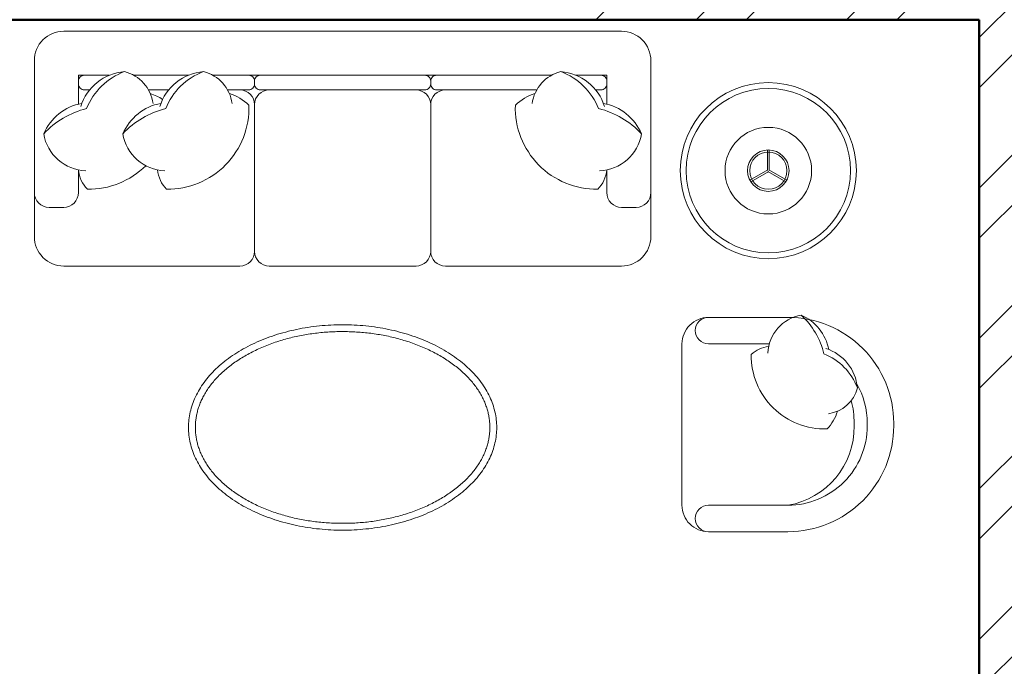
# Model space of a CAD drawing. Units: inches. Extents: x 1901 to 2863, y 888 to 2433.
# Tile 38 of 91: x 2530 to 2618, y 1603 to 1661. Entities that reach past the tile are written whole.
import ezdxf

# ---------------------------------------------------------------- set-up
doc = ezdxf.new("R2010")
doc.units = ezdxf.units.IN
for name, color, linetype, lineweight in [('A-FURN', 8, 'Continuous', 18), ('A-WALL', 7, 'Continuous', 50), ('A-WALL-PATT', 8, 'Continuous', 13)]:
    doc.layers.add(name, color=color, linetype=linetype, lineweight=lineweight)

msp = doc.modelspace()

# ---------------------------------------------------------------- hatches: boundary and pattern name
at = {"layer": 'A-WALL-PATT'}
h = msp.add_hatch(dxfattribs=at)
h.set_pattern_fill('ANSI32', color=256)
h.paths.add_polyline_path([(2443.926, 2139.888), (2439.426, 2139.888), (2439.426, 2069.348), (2441.676, 2069.348), (2443.926, 2069.348), (2443.926, 2078.634), (2521.926, 2078.634), (2521.926, 2075.067), (2524.176, 2075.067), (2526.426, 2075.067), (2526.426, 2078.634), (2571.755, 2078.634), (2571.755, 2080.884), (2571.755, 2083.134), (2443.926, 2083.134)])
h.paths.add_polyline_path([(2526.426, 2054.634), (2524.176, 2054.634), (2521.926, 2054.634), (2521.926, 2030.634), (2443.926, 2030.634), (2443.926, 2045.348), (2439.426, 2045.348), (2439.426, 1983.867), (2443.926, 1983.867), (2443.926, 2026.134), (2521.926, 2026.134), (2526.426, 2026.134)])
h.paths.add_polyline_path([(2443.926, 1923.867), (2439.426, 1923.867), (2439.426, 1872.634), (2443.926, 1872.634)])
h.paths.add_polyline_path([(2636.233, 1766.134), (2609.926, 1766.134), (2609.926, 1779.785), (2605.426, 1779.785), (2605.426, 1766.134), (2486.614, 1766.134), (2486.614, 1770.671), (2482.114, 1770.671), (2482.114, 1766.134), (2482.114, 1761.634), (2636.233, 1761.634), (2636.233, 1763.884)])
h.paths.add_polyline_path([(2519.536, 1663.384), (2519.536, 1665.634), (2494.926, 1665.634), (2481.831, 1665.634), (2481.831, 1663.384), (2481.831, 1661.134), (2490.426, 1661.134), (2490.426, 1640.157), (2494.926, 1640.157), (2494.926, 1661.134), (2519.536, 1661.134)])
h.paths.add_polyline_path([(2443.926, 1712.134), (2443.926, 1716.634), (2414.464, 1716.634), (2414.464, 1712.134), (2439.426, 1712.134), (2439.426, 1545.507), (2443.926, 1545.507), (2443.926, 1661.134), (2448.475, 1661.134), (2448.475, 1665.634), (2443.926, 1665.634)])
h.paths.add_polyline_path([(2343.426, 1712.134), (2365.525, 1712.134), (2365.525, 1714.384), (2365.525, 1716.634), (2333.871, 1716.634), (2333.871, 1714.384), (2333.871, 1712.134), (2338.926, 1712.134), (2338.926, 1575.634), (2338.926, 1545.507), (2343.426, 1545.507), (2343.426, 1547.507), (2343.426, 1580.134)])
h.paths.add_polyline_path([(2752.926, 1665.634), (2579.536, 1665.634), (2579.536, 1661.134), (2615.926, 1661.134), (2615.926, 1529.134), (2598.931, 1529.134), (2598.931, 1524.634), (2623.127, 1524.634), (2623.127, 1526.884), (2623.127, 1529.134), (2620.426, 1529.134), (2620.426, 1661.134), (2748.426, 1661.134), (2748.426, 1633.499), (2752.926, 1633.499)])
h.paths.add_polyline_path([(2752.926, 1419.929), (2748.426, 1419.929), (2748.426, 1400.134), (2659.426, 1400.134), (2659.426, 1444.333), (2657.176, 1444.333), (2654.926, 1444.333), (2654.926, 1400.134), (2643.649, 1400.134), (2643.649, 1395.634), (2748.426, 1395.634), (2748.426, 1364.035), (2752.926, 1364.035)])
h.paths.add_polyline_path([(2752.926, 1492.878), (2748.426, 1492.878), (2748.426, 1476.634), (2667.426, 1476.634), (2667.426, 1479.71), (2665.176, 1479.71), (2662.926, 1479.71), (2662.926, 1476.634), (2654.926, 1476.634), (2654.926, 1469.536), (2659.426, 1469.536), (2659.426, 1472.134), (2748.426, 1472.134), (2748.426, 1455.929), (2752.926, 1455.929)])
h.paths.add_polyline_path([(2752.926, 1304.035), (2748.426, 1304.035), (2748.426, 1263.634), (2738.66, 1263.634), (2738.66, 1259.134), (2752.926, 1259.134)])
h.paths.add_polyline_path([(2685.926, 1259.134), (2695.49, 1259.134), (2695.49, 1261.384), (2695.49, 1263.634), (2677.837, 1263.634), (2677.837, 1261.384), (2677.837, 1259.134), (2681.426, 1259.134), (2681.426, 1203.634), (2653.277, 1203.634), (2653.277, 1199.134), (2685.926, 1199.134), (2685.926, 1203.634)])
h.paths.add_polyline_path([(2609.426, 1395.634), (2611.848, 1395.634), (2611.848, 1400.134), (2598.888, 1400.134), (2598.888, 1397.884), (2598.888, 1395.634), (2604.926, 1395.634), (2604.926, 1268.134), (2554.726, 1268.134), (2554.726, 1265.884), (2554.726, 1263.634), (2604.926, 1263.634), (2604.926, 1203.634), (2571.306, 1203.634), (2571.306, 1199.134), (2604.926, 1199.134), (2629.277, 1199.134), (2629.277, 1201.384), (2629.277, 1203.634), (2609.426, 1203.634), (2609.426, 1258.634), (2609.426, 1259.134), (2654.804, 1259.134), (2654.804, 1263.634), (2609.426, 1263.634)])
h.paths.add_polyline_path([(2443.926, 1304.035), (2439.426, 1304.035), (2439.426, 1259.134), (2443.926, 1259.134), (2456.16, 1259.134), (2456.16, 1261.384), (2456.16, 1263.634), (2443.926, 1263.634)])
h.paths.add_polyline_path([(2525.426, 1263.634), (2531.778, 1263.634), (2531.778, 1268.134), (2520.926, 1268.134), (2520.926, 1263.634), (2511.409, 1263.634), (2511.409, 1259.134), (2520.926, 1259.134), (2520.926, 1199.134), (2547.306, 1199.134), (2547.306, 1201.384), (2547.306, 1203.634), (2525.426, 1203.634)])
h.paths.add_polyline_path([(2443.926, 1434.842), (2439.426, 1434.842), (2439.426, 1364.035), (2441.676, 1364.035), (2443.926, 1364.035)])
h.paths.add_polyline_path([(2567.134, 1400.134), (2443.926, 1400.134), (2443.926, 1395.634), (2567.134, 1395.634)])
h.paths.add_polyline_path([(2443.926, 1545.507), (2439.426, 1545.507), (2439.426, 1494.842), (2443.926, 1494.842)])
h.paths.add_polyline_path([(2494.926, 1553.349), (2492.676, 1553.349), (2490.426, 1553.349), (2490.426, 1524.634), (2494.926, 1524.634), (2525.936, 1524.634), (2525.936, 1526.884), (2525.936, 1529.134), (2494.926, 1529.134)])
h.paths.add_polyline_path([(2752.926, 1573.499), (2748.426, 1573.499), (2748.426, 1529.134), (2657.759, 1529.134), (2657.759, 1524.634), (2662.926, 1524.634), (2662.926, 1498.631), (2667.426, 1498.631), (2667.426, 1524.634), (2748.426, 1524.634), (2748.426, 1516.878), (2752.926, 1516.878)])
h.paths.add_polyline_path([(2038.602, 2237.418), (2080.174, 2237.418), (2080.174, 2256.075), (2038.602, 2256.075)], flags=9)
h.paths.add_polyline_path([(2292.009, 1062.394), (2539.932, 1062.394), (2539.932, 1099.487), (2292.009, 1099.487)], flags=9)
h.paths.add_polyline_path([(2424.91, 1832.253), (2448.513, 1832.253), (2448.513, 1846.678), (2424.91, 1846.678)], flags=9)
h.paths.add_polyline_path([(2359.076, 1832.253), (2382.678, 1832.253), (2382.678, 1846.678), (2359.076, 1846.678)], flags=9)
h.paths.add_polyline_path([(2352.899, 1684.802), (2367.543, 1684.802), (2367.543, 1697.167), (2352.899, 1697.167)], flags=9)
h.paths.add_polyline_path([(2079.288, 1755.826), (2169.024, 1755.826), (2169.024, 1774.372), (2079.288, 1774.372)], flags=9)
h.paths.add_polyline_path([(2404.09, 1373.857), (2404.09, 1463.593), (2385.544, 1463.593), (2385.544, 1373.857)], flags=9)
h.paths.add_polyline_path([(2268.091, 2236.371), (2309.636, 2236.371), (2309.636, 2255.028), (2268.091, 2255.028)], flags=9)
h.paths.add_polyline_path([(2575.96, 1700.951), (2665.696, 1700.951), (2665.696, 1719.498), (2575.96, 1719.498)], flags=9)
h.paths.add_polyline_path([(2302.962, 1878.474), (2329.524, 1878.474), (2329.524, 1888.777), (2302.962, 1888.777)], flags=9)
h.paths.add_polyline_path([(2097.415, 2240.576), (2126.573, 2240.576), (2126.573, 2259.233), (2097.415, 2259.233)], flags=9)
h.paths.add_polyline_path([(2208.725, 2246.124), (2237.882, 2246.124), (2237.882, 2264.781), (2208.725, 2264.781)], flags=9)
h.paths.add_polyline_path([(2038.147, 1925.958), (2076.987, 1925.958), (2076.987, 1944.615), (2038.147, 1944.615)], flags=9)
h.paths.add_polyline_path([(2239.144, 1926.672), (2288.465, 1926.672), (2288.465, 1945.329), (2239.144, 1945.329)], flags=9)
h.paths.add_polyline_path([(2175.429, 2007.33), (2212.356, 2007.33), (2212.356, 2025.987), (2175.429, 2025.987)], flags=9)
h.paths.add_polyline_path([(2225.034, 2091.794), (2263.875, 2091.794), (2263.875, 2110.451), (2225.034, 2110.451)], flags=9)
h.paths.add_polyline_path([(2035.398, 2098.478), (2074.238, 2098.478), (2074.238, 2117.135), (2035.398, 2117.135)], flags=9)
h.paths.add_polyline_path([(2050.102, 2029.209), (2083.26, 2029.209), (2083.26, 2047.866), (2050.102, 2047.866)], flags=9)
h.paths.add_polyline_path([(2069.677, 1956.719), (2098.835, 1956.719), (2098.835, 1975.376), (2069.677, 1975.376)], flags=9)
h.paths.add_polyline_path([(2328.62, 1753.336), (2361.663, 1753.336), (2361.663, 1771.993), (2328.62, 1771.993)], flags=9)
h.paths.add_polyline_path([(2395.162, 2060.888), (2395.162, 2140.654), (2378.676, 2140.654), (2378.676, 2060.888)], flags=9)
h.paths.add_polyline_path([(2463.728, 2059.02), (2492.886, 2059.02), (2492.886, 2077.677), (2463.728, 2077.677)], flags=9)
h.paths.add_polyline_path([(2458.027, 2181.536), (2496.868, 2181.536), (2496.868, 2200.194), (2458.027, 2200.194)], flags=9)
h.paths.add_polyline_path([(2456.855, 2228.831), (2498.401, 2228.831), (2498.401, 2247.488), (2456.855, 2247.488)], flags=9)
h.paths.add_polyline_path([(2527.577, 2243.074), (2556.735, 2243.074), (2556.735, 2261.731), (2527.577, 2261.731)], flags=9)
h.paths.add_polyline_path([(2694.461, 2232.767), (2736.033, 2232.767), (2736.033, 2251.425), (2694.461, 2251.425)], flags=9)
h.paths.add_polyline_path([(2637.821, 2249.225), (2666.979, 2249.225), (2666.979, 2267.882), (2637.821, 2267.882)], flags=9)
h.paths.add_polyline_path([(2623.687, 2183.541), (2662.528, 2183.541), (2662.528, 2202.199), (2623.687, 2202.199)], flags=9)
h.paths.add_polyline_path([(2691.965, 2021.5), (2725.124, 2021.5), (2725.124, 2040.157), (2691.965, 2040.157)], flags=9)
h.paths.add_polyline_path([(2621.043, 1975.912), (2662.335, 1975.912), (2662.335, 1994.569), (2621.043, 1994.569)], flags=9)
h.paths.add_polyline_path([(2479.032, 1927.62), (2519.844, 1927.62), (2519.844, 1946.277), (2479.032, 1946.277)], flags=9)
h.paths.add_polyline_path([(2670.941, 1849.076), (2716.005, 1849.076), (2716.005, 1867.734), (2670.941, 1867.734)], flags=9)
h.paths.add_polyline_path([(2523.613, 1782.956), (2550.175, 1782.956), (2550.175, 1793.26), (2523.613, 1793.26)], flags=9)
h.paths.add_polyline_path([(2450.841, 1207.331), (2492.386, 1207.331), (2492.386, 1225.989), (2450.841, 1225.989)], flags=9)
h.paths.add_polyline_path([(2527.751, 1203.841), (2556.908, 1203.841), (2556.908, 1222.499), (2527.751, 1222.499)], flags=9)
h.paths.add_polyline_path([(2639.111, 1207.2), (2668.268, 1207.2), (2668.268, 1225.857), (2639.111, 1225.857)], flags=9)
h.paths.add_polyline_path([(2692.594, 1218.965), (2734.167, 1218.965), (2734.167, 1237.623), (2692.594, 1237.623)], flags=9)
h.paths.add_polyline_path([(2669.266, 1366.329), (2708.106, 1366.329), (2708.106, 1384.987), (2669.266, 1384.987)], flags=25)
h.paths.add_polyline_path([(2463.313, 1358.031), (2502.153, 1358.031), (2502.153, 1376.688), (2463.313, 1376.688)], flags=9)
h.paths.add_polyline_path([(2494.725, 1449.963), (2531.652, 1449.963), (2531.652, 1468.62), (2494.725, 1468.62)], flags=9)
h.paths.add_polyline_path([(2675.565, 1422.157), (2708.724, 1422.157), (2708.724, 1440.815), (2675.565, 1440.815)], flags=25)
h.paths.add_polyline_path([(2685.634, 1493.891), (2714.792, 1493.891), (2714.792, 1512.548), (2685.634, 1512.548)], flags=9)
h.paths.add_polyline_path([(2686.805, 1529.913), (2725.645, 1529.913), (2725.645, 1548.57), (2686.805, 1548.57)], flags=25)
h.paths.add_polyline_path([(2503.651, 1537.991), (2552.972, 1537.991), (2552.972, 1556.648), (2503.651, 1556.648)], flags=9)
h.paths.add_polyline_path([(2291.713, 1643.504), (2318.275, 1643.504), (2318.275, 1653.807), (2291.713, 1653.807)], flags=9)
h.paths.add_polyline_path([(2450.626, 1610.52), (2477.189, 1610.52), (2477.189, 1620.824), (2450.626, 1620.824)], flags=9)
h.paths.add_polyline_path([(2359.985, 1551.814), (2422.253, 1551.814), (2422.253, 1562.117), (2359.985, 1562.117)], flags=9)
h.paths.add_polyline_path([(2280.106, 1249.006), (2321.651, 1249.006), (2321.651, 1267.663), (2280.106, 1267.663)], flags=9)
h.paths.add_polyline_path([(2164.057, 1274.232), (2193.215, 1274.232), (2193.215, 1292.889), (2164.057, 1292.889)], flags=9)
h.paths.add_polyline_path([(2118.21, 1277.694), (2151.252, 1277.694), (2151.252, 1296.351), (2118.21, 1296.351)], flags=9)
h.paths.add_polyline_path([(2031.946, 1268.529), (2073.519, 1268.529), (2073.519, 1287.187), (2031.946, 1287.187)], flags=9)
h.paths.add_polyline_path([(2050.199, 1409.079), (2089.04, 1409.079), (2089.04, 1427.736), (2050.199, 1427.736)], flags=9)
h.paths.add_polyline_path([(2243.743, 1421.032), (2282.584, 1421.032), (2282.584, 1439.689), (2243.743, 1439.689)], flags=9)
h.paths.add_polyline_path([(2190.746, 1509.769), (2231.558, 1509.769), (2231.558, 1528.426), (2190.746, 1528.426)], flags=9)
h.paths.add_polyline_path([(2058.392, 1475.415), (2091.55, 1475.415), (2091.55, 1494.073), (2058.392, 1494.073)], flags=9)
h.paths.add_polyline_path([(2062.447, 1553.09), (2091.605, 1553.09), (2091.605, 1571.747), (2062.447, 1571.747)], flags=9)
h.paths.add_polyline_path([(2219.524, 1590.365), (2266.147, 1590.365), (2266.147, 1609.022), (2219.524, 1609.022)], flags=9)
h.paths.add_polyline_path([(2041.072, 1584.188), (2079.912, 1584.188), (2079.912, 1602.845), (2041.072, 1602.845)], flags=9)

# ---------------------------------------------------------------- linework, layer by layer
at = {"layer": 'A-FURN', "ltscale": 0.03}
for p, q in [((2596.965, 1647.616), (2596.965, 1649.469)), ((2597.131, 1647.616), (2597.131, 1649.469)), ((2597.007, 1647.687), (2595.402, 1646.761)), ((2597.089, 1647.544), (2595.485, 1646.617)), ((2597.007, 1647.544), (2598.611, 1646.617)), ((2597.089, 1647.687), (2598.694, 1646.761))]:
    msp.add_line(p, q, dxfattribs=at)
msp.add_lwpolyline([(2586.536, 1641.703, -0.414214), (2583.908, 1639.075), (2568.14, 1639.075, -0.414214), (2566.826, 1640.389, -0.414214), (2565.512, 1639.075), (2552.372, 1639.075, -0.414214), (2551.058, 1640.389, -0.414214), (2549.744, 1639.075), (2533.976, 1639.075, -0.414214), (2531.348, 1641.703), (2531.348, 1657.471, -0.414214), (2533.976, 1660.099), (2583.908, 1660.099, -0.414214), (2586.536, 1657.471)], format="xyb", close=True, dxfattribs=at)
at = {"layer": 'A-FURN'}
for points in [[(2532.184, 1650.913, -0.14773), (2536.025, 1653.171, -0.213343), (2539.413, 1656.483, -0.178662)], [(2535.494, 1653.351, -0.306663), (2539.413, 1656.483, -0.30633), (2541.974, 1653.623, 0.872847)], [(2539.263, 1650.913, -0.14773), (2543.103, 1653.171, -0.213343), (2546.492, 1656.483, -0.178662)], [(2542.573, 1653.351, -0.306663), (2546.492, 1656.483, -0.30633), (2549.052, 1653.623, 0.872847)], [(2582.39, 1653.351, 0.306663), (2578.471, 1656.483, 0.30633), (2575.91, 1653.623, -0.872847)], [(2585.7, 1650.913, 0.14773), (2581.859, 1653.171, 0.213343), (2578.471, 1656.483, 0.178662)], [(2538.054, 1656.157), (2535.29, 1656.157), (2535.29, 1653.574, -0.414214)], [(2536.293, 1654.843), (2535.816, 1654.843, -0.414214), (2535.29, 1655.368), (2535.29, 1655.631, -0.414214), (2535.816, 1656.157)], [(2535.816, 1656.157), (2538.054, 1656.157, -0.414214)], [(2540.24, 1656.157), (2545.133, 1656.157, -0.414214)], [(2547.319, 1656.157), (2550.532, 1656.157, -0.414214), (2551.058, 1655.631), (2551.058, 1655.368, -0.414214), (2550.532, 1654.843), (2548.642, 1654.843, -0.414214)], [(2577.644, 1656.157), (2567.352, 1656.157, 0.414214), (2566.826, 1655.631), (2566.826, 1655.368, 0.414214), (2567.352, 1654.843), (2576.321, 1654.843, 0.414214)], [(2582.068, 1656.157), (2579.83, 1656.157, 0.414214)], [(2581.591, 1654.843), (2582.068, 1654.843, 0.414214), (2582.594, 1655.368), (2582.594, 1655.631, 0.414214), (2582.068, 1656.157)], [(2543.371, 1654.843), (2541.563, 1654.843, -0.414214)], [(2542.83, 1653.996, 0.071865), (2541.728, 1654.51, -7.115464)], [(2542.366, 1647.681, 0.165541), (2543.179, 1645.945, 0.425989), (2550.558, 1653.472, 0.121523), (2548.806, 1654.51, -7.115464)], [(2549.744, 1654.843, -0.414214), (2551.058, 1653.529), (2551.058, 1640.389, -0.414214)], [(2552.372, 1654.843, 0.414214), (2551.058, 1653.529)], [(2565.512, 1654.843, -0.414214), (2566.826, 1653.529)], [(2568.14, 1654.843, 0.414214), (2566.826, 1653.529), (2566.826, 1640.389, 0.414214)], [(2582.597, 1647.681, -0.165541), (2581.784, 1645.945, -0.425989), (2574.404, 1653.472, -0.121523), (2576.156, 1654.51, 7.115464)], [(2535.949, 1647.601, -0.356772), (2532.184, 1650.913, -0.249542), (2535.596, 1653.642, 9.61688)], [(2543.028, 1647.601, -0.356772), (2539.263, 1650.913, -0.249542), (2542.674, 1653.642, 9.61688)], [(2581.935, 1647.601, 0.356772), (2585.7, 1650.913, 0.249542), (2582.288, 1653.642, -9.61688)], [(2535.29, 1647.68), (2535.29, 1645.645, -0.414214), (2533.976, 1644.331), (2532.662, 1644.331, -0.414214), (2531.348, 1645.645)], [(2535.287, 1647.681, 0.165541), (2536.1, 1645.945, 0.200231), (2541.316, 1648.059, 0.121523)], [(2586.536, 1645.645, -0.414214), (2585.222, 1644.331), (2583.908, 1644.331, -0.414214), (2582.594, 1645.645), (2582.594, 1647.68)], [(2597.14, 1632.11), (2591.693, 1632.11, -0.414214), (2590.508, 1633.295), (2590.508, 1633.295, -0.414214), (2591.693, 1634.48)], [(2597.011, 1631.279, -0.356772), (2599.997, 1634.674, -0.249542), (2602.458, 1631.598, 9.61688)], [(2599.997, 1634.674, -0.14773), (2602.033, 1631.211, -0.213343), (2605.02, 1628.156, -0.178662)], [(2597.083, 1631.876, 0.165541), (2595.518, 1631.143, 0.425989), (2602.305, 1624.489, 0.121523), (2603.24, 1626.069, -7.115464)], [(2602.196, 1631.689, -0.306663), (2605.02, 1628.156, -0.30633), (2602.441, 1625.847, 0.872847)], [(2604.972, 1628.53, -0.130591), (2605.91, 1625.002), (2605.91, 1624.883)], [(2604.47, 1627.022, -0.072384), (2604.725, 1625.002), (2604.725, 1624.883)], [(2598.801, 1617.656, 0.372719), (2604.725, 1624.765), (2604.725, 1624.883)], [(2598.801, 1617.656, 0.414214), (2605.91, 1624.765), (2605.91, 1624.883)], [(2598.802, 1617.656), (2591.693, 1617.656, 0.414214), (2590.508, 1616.472), (2590.508, 1616.472, 0.414214), (2591.693, 1615.287)]]:
    msp.add_lwpolyline(points, format="xyb", dxfattribs=at)
for points in [[(2545.133, 1656.157), (2540.24, 1656.157)], [(2577.644, 1656.157), (2547.319, 1656.157)], [(2582.594, 1653.574), (2582.594, 1656.157), (2579.83, 1656.157)]]:
    msp.add_lwpolyline(points, dxfattribs=at)
msp.add_lwpolyline([(2551.584, 1656.157), (2566.3, 1656.157, -0.414214), (2566.826, 1655.631), (2566.826, 1655.368, -0.414214), (2566.3, 1654.843), (2551.584, 1654.843, -0.414214), (2551.058, 1655.368), (2551.058, 1655.631, -0.414214)], format="xyb", close=True, dxfattribs=at)
at = {"layer": 'A-FURN', "ltscale": 0.03}
msp.add_lwpolyline([(2589.323, 1624.883), (2589.323, 1617.656, 0.414214), (2591.693, 1615.287), (2598.801, 1615.287, 0.414214), (2608.279, 1624.765), (2608.279, 1624.883), (2608.279, 1625.002, 0.414214), (2598.801, 1634.48), (2591.693, 1634.48, 0.414214), (2589.323, 1632.11), (2589.323, 1624.883)], format="xyb", dxfattribs=at)
msp.add_polyline3d([(2572.739, 1624.621, 0), (2572.737, 1624.795, 0), (2572.729, 1624.969, 0), (2572.717, 1625.143, 0), (2572.7, 1625.316, 0), (2572.677, 1625.49, 0), (2572.65, 1625.663, 0), (2572.618, 1625.836, 0), (2572.581, 1626.008, 0), (2572.539, 1626.18, 0), (2572.493, 1626.351, 0), (2572.441, 1626.522, 0), (2572.385, 1626.692, 0), (2572.324, 1626.861, 0), (2572.258, 1627.029, 0), (2572.187, 1627.197, 0), (2572.111, 1627.363, 0), (2572.031, 1627.529, 0), (2571.946, 1627.694, 0), (2571.857, 1627.857, 0), (2571.762, 1628.02, 0), (2571.664, 1628.181, 0), (2571.56, 1628.341, 0), (2571.452, 1628.499, 0), (2571.34, 1628.656, 0), (2571.223, 1628.812, 0), (2571.102, 1628.966, 0), (2570.977, 1629.119, 0), (2570.847, 1629.27, 0), (2570.713, 1629.419, 0), (2570.574, 1629.567, 0), (2570.432, 1629.713, 0), (2570.285, 1629.857, 0), (2570.135, 1629.999, 0), (2569.98, 1630.139, 0), (2569.821, 1630.277, 0), (2569.659, 1630.414, 0), (2569.492, 1630.548, 0), (2569.322, 1630.68, 0), (2569.148, 1630.81, 0), (2568.971, 1630.937, 0), (2568.79, 1631.063, 0), (2568.605, 1631.186, 0), (2568.417, 1631.307, 0), (2568.226, 1631.425, 0), (2568.031, 1631.541, 0), (2567.833, 1631.654, 0), (2567.632, 1631.765, 0), (2567.427, 1631.874, 0), (2567.22, 1631.979, 0), (2567.009, 1632.082, 0), (2566.796, 1632.183, 0), (2566.58, 1632.281, 0), (2566.361, 1632.376, 0), (2566.14, 1632.468, 0), (2565.916, 1632.557, 0), (2565.689, 1632.644, 0), (2565.46, 1632.727, 0), (2565.229, 1632.808, 0), (2564.995, 1632.886, 0), (2564.76, 1632.961, 0), (2564.522, 1633.033, 0), (2564.282, 1633.102, 0), (2564.04, 1633.168, 0), (2563.797, 1633.23, 0), (2563.552, 1633.29, 0), (2563.305, 1633.347, 0), (2563.056, 1633.4, 0), (2562.806, 1633.45, 0), (2562.555, 1633.498, 0), (2562.302, 1633.542, 0), (2562.049, 1633.582, 0), (2561.794, 1633.62, 0), (2561.538, 1633.654, 0), (2561.281, 1633.686, 0), (2561.023, 1633.713, 0), (2560.764, 1633.738, 0), (2560.505, 1633.759, 0), (2560.246, 1633.777, 0), (2559.985, 1633.792, 0), (2559.725, 1633.804, 0), (2559.464, 1633.812, 0), (2559.203, 1633.817, 0), (2558.942, 1633.819, 0), (2558.681, 1633.817, 0), (2558.42, 1633.812, 0), (2558.159, 1633.804, 0), (2557.899, 1633.792, 0), (2557.638, 1633.777, 0), (2557.379, 1633.759, 0), (2557.12, 1633.738, 0), (2556.861, 1633.713, 0), (2556.603, 1633.686, 0), (2556.346, 1633.654, 0), (2556.091, 1633.62, 0), (2555.836, 1633.582, 0), (2555.582, 1633.542, 0), (2555.329, 1633.498, 0), (2555.078, 1633.45, 0), (2554.828, 1633.4, 0), (2554.579, 1633.347, 0), (2554.332, 1633.29, 0), (2554.087, 1633.23, 0), (2553.844, 1633.168, 0), (2553.602, 1633.102, 0), (2553.362, 1633.033, 0), (2553.124, 1632.961, 0), (2552.889, 1632.886, 0), (2552.655, 1632.808, 0), (2552.424, 1632.727, 0), (2552.195, 1632.644, 0), (2551.968, 1632.557, 0), (2551.744, 1632.468, 0), (2551.523, 1632.376, 0), (2551.304, 1632.281, 0), (2551.088, 1632.183, 0), (2550.875, 1632.082, 0), (2550.664, 1631.979, 0), (2550.457, 1631.874, 0), (2550.253, 1631.765, 0), (2550.051, 1631.654, 0), (2549.853, 1631.541, 0), (2549.658, 1631.425, 0), (2549.467, 1631.307, 0), (2549.279, 1631.186, 0), (2549.094, 1631.063, 0), (2548.913, 1630.937, 0), (2548.736, 1630.81, 0), (2548.562, 1630.68, 0), (2548.392, 1630.548, 0), (2548.225, 1630.414, 0), (2548.063, 1630.277, 0), (2547.904, 1630.139, 0), (2547.749, 1629.999, 0), (2547.599, 1629.857, 0), (2547.452, 1629.713, 0), (2547.31, 1629.567, 0), (2547.171, 1629.419, 0), (2547.037, 1629.27, 0), (2546.907, 1629.119, 0), (2546.782, 1628.966, 0), (2546.661, 1628.812, 0), (2546.544, 1628.656, 0), (2546.432, 1628.499, 0), (2546.324, 1628.341, 0), (2546.22, 1628.181, 0), (2546.122, 1628.02, 0), (2546.027, 1627.857, 0), (2545.938, 1627.694, 0), (2545.853, 1627.529, 0), (2545.773, 1627.363, 0), (2545.697, 1627.197, 0), (2545.626, 1627.029, 0), (2545.56, 1626.861, 0), (2545.499, 1626.692, 0), (2545.443, 1626.522, 0), (2545.391, 1626.351, 0), (2545.345, 1626.18, 0), (2545.303, 1626.008, 0), (2545.266, 1625.836, 0), (2545.234, 1625.663, 0), (2545.207, 1625.49, 0), (2545.185, 1625.316, 0), (2545.167, 1625.143, 0), (2545.155, 1624.969, 0), (2545.148, 1624.795, 0), (2545.145, 1624.621, 0), (2545.148, 1624.447, 0), (2545.155, 1624.273, 0), (2545.167, 1624.099, 0), (2545.185, 1623.925, 0), (2545.207, 1623.752, 0), (2545.234, 1623.578, 0), (2545.266, 1623.406, 0), (2545.303, 1623.233, 0), (2545.345, 1623.062, 0), (2545.391, 1622.89, 0), (2545.443, 1622.72, 0), (2545.499, 1622.55, 0), (2545.56, 1622.38, 0), (2545.626, 1622.212, 0), (2545.697, 1622.044, 0), (2545.773, 1621.878, 0), (2545.853, 1621.712, 0), (2545.938, 1621.548, 0), (2546.027, 1621.384, 0), (2546.122, 1621.222, 0), (2546.22, 1621.061, 0), (2546.324, 1620.901, 0), (2546.432, 1620.742, 0), (2546.544, 1620.585, 0), (2546.661, 1620.429, 0), (2546.782, 1620.275, 0), (2546.907, 1620.122, 0), (2547.037, 1619.971, 0), (2547.171, 1619.822, 0), (2547.31, 1619.674, 0), (2547.452, 1619.529, 0), (2547.599, 1619.385, 0), (2547.749, 1619.242, 0), (2547.904, 1619.102, 0), (2548.063, 1618.964, 0), (2548.225, 1618.828, 0), (2548.392, 1618.693, 0), (2548.562, 1618.561, 0), (2548.736, 1618.432, 0), (2548.913, 1618.304, 0), (2549.094, 1618.178, 0), (2549.279, 1618.055, 0), (2549.467, 1617.935, 0), (2549.658, 1617.816, 0), (2549.853, 1617.7, 0), (2550.051, 1617.587, 0), (2550.253, 1617.476, 0), (2550.457, 1617.368, 0), (2550.664, 1617.262, 0), (2550.875, 1617.159, 0), (2551.088, 1617.058, 0), (2551.304, 1616.961, 0), (2551.523, 1616.866, 0), (2551.744, 1616.773, 0), (2551.968, 1616.684, 0), (2552.195, 1616.598, 0), (2552.424, 1616.514, 0), (2552.655, 1616.433, 0), (2552.889, 1616.355, 0), (2553.124, 1616.28, 0), (2553.362, 1616.208, 0), (2553.602, 1616.14, 0), (2553.844, 1616.074, 0), (2554.087, 1616.011, 0), (2554.332, 1615.951, 0), (2554.579, 1615.895, 0), (2554.828, 1615.841, 0), (2555.078, 1615.791, 0), (2555.329, 1615.744, 0), (2555.582, 1615.7, 0), (2555.836, 1615.659, 0), (2556.091, 1615.621, 0), (2556.346, 1615.587, 0), (2556.603, 1615.556, 0), (2556.861, 1615.528, 0), (2557.12, 1615.503, 0), (2557.379, 1615.482, 0), (2557.638, 1615.464, 0), (2557.899, 1615.449, 0), (2558.159, 1615.437, 0), (2558.42, 1615.429, 0), (2558.681, 1615.424, 0), (2558.942, 1615.423, 0), (2559.203, 1615.424, 0), (2559.464, 1615.429, 0), (2559.725, 1615.437, 0), (2559.985, 1615.449, 0), (2560.246, 1615.464, 0), (2560.505, 1615.482, 0), (2560.764, 1615.503, 0), (2561.023, 1615.528, 0), (2561.281, 1615.556, 0), (2561.538, 1615.587, 0), (2561.794, 1615.621, 0), (2562.049, 1615.659, 0), (2562.302, 1615.7, 0), (2562.555, 1615.744, 0), (2562.806, 1615.791, 0), (2563.056, 1615.841, 0), (2563.305, 1615.895, 0), (2563.552, 1615.951, 0), (2563.797, 1616.011, 0), (2564.04, 1616.074, 0), (2564.282, 1616.14, 0), (2564.522, 1616.208, 0), (2564.76, 1616.28, 0), (2564.995, 1616.355, 0), (2565.229, 1616.433, 0), (2565.46, 1616.514, 0), (2565.689, 1616.598, 0), (2565.916, 1616.684, 0), (2566.14, 1616.773, 0), (2566.361, 1616.866, 0), (2566.58, 1616.961, 0), (2566.796, 1617.058, 0), (2567.009, 1617.159, 0), (2567.22, 1617.262, 0), (2567.427, 1617.368, 0), (2567.632, 1617.476, 0), (2567.833, 1617.587, 0), (2568.031, 1617.7, 0), (2568.226, 1617.816, 0), (2568.417, 1617.935, 0), (2568.605, 1618.055, 0), (2568.79, 1618.178, 0), (2568.971, 1618.304, 0), (2569.148, 1618.432, 0), (2569.322, 1618.561, 0), (2569.492, 1618.693, 0), (2569.659, 1618.828, 0), (2569.821, 1618.964, 0), (2569.98, 1619.102, 0), (2570.135, 1619.242, 0), (2570.285, 1619.385, 0), (2570.432, 1619.529, 0), (2570.574, 1619.674, 0), (2570.713, 1619.822, 0), (2570.847, 1619.971, 0), (2570.977, 1620.122, 0), (2571.102, 1620.275, 0), (2571.223, 1620.429, 0), (2571.34, 1620.585, 0), (2571.452, 1620.742, 0), (2571.56, 1620.901, 0), (2571.664, 1621.061, 0), (2571.762, 1621.222, 0), (2571.857, 1621.384, 0), (2571.946, 1621.548, 0), (2572.031, 1621.712, 0), (2572.111, 1621.878, 0), (2572.187, 1622.044, 0), (2572.258, 1622.212, 0), (2572.324, 1622.38, 0), (2572.385, 1622.55, 0), (2572.441, 1622.72, 0), (2572.493, 1622.89, 0), (2572.539, 1623.062, 0), (2572.581, 1623.233, 0), (2572.618, 1623.406, 0), (2572.65, 1623.578, 0), (2572.677, 1623.752, 0), (2572.7, 1623.925, 0), (2572.717, 1624.099, 0), (2572.729, 1624.273, 0), (2572.737, 1624.447, 0), (2572.739, 1624.621, 0)], dxfattribs=at)
at = {"layer": 'A-FURN'}
msp.add_polyline3d([(2572.126, 1624.621, 0), (2572.125, 1624.715, 0), (2572.123, 1624.809, 0), (2572.119, 1624.904, 0), (2572.113, 1624.999, 0), (2572.105, 1625.095, 0), (2572.096, 1625.191, 0), (2572.085, 1625.288, 0), (2572.073, 1625.385, 0), (2572.058, 1625.482, 0), (2572.042, 1625.579, 0), (2572.024, 1625.677, 0), (2572.005, 1625.775, 0), (2571.983, 1625.874, 0), (2571.959, 1625.972, 0), (2571.934, 1626.071, 0), (2571.907, 1626.17, 0), (2571.877, 1626.27, 0), (2571.846, 1626.37, 0), (2571.813, 1626.469, 0), (2571.777, 1626.57, 0), (2571.74, 1626.67, 0), (2571.701, 1626.77, 0), (2571.659, 1626.871, 0), (2571.616, 1626.971, 0), (2571.57, 1627.072, 0), (2571.523, 1627.173, 0), (2571.473, 1627.273, 0), (2571.421, 1627.374, 0), (2571.367, 1627.475, 0), (2571.311, 1627.575, 0), (2571.253, 1627.676, 0), (2571.193, 1627.776, 0), (2571.13, 1627.876, 0), (2571.066, 1627.976, 0), (2570.999, 1628.076, 0), (2570.93, 1628.175, 0), (2570.859, 1628.274, 0), (2570.786, 1628.373, 0), (2570.711, 1628.472, 0), (2570.634, 1628.57, 0), (2570.555, 1628.667, 0), (2570.473, 1628.765, 0), (2570.389, 1628.861, 0), (2570.303, 1628.958, 0), (2570.215, 1629.053, 0), (2570.124, 1629.148, 0), (2570.031, 1629.243, 0), (2569.936, 1629.337, 0), (2569.839, 1629.431, 0), (2569.74, 1629.523, 0), (2569.639, 1629.615, 0), (2569.535, 1629.707, 0), (2569.43, 1629.798, 0), (2569.323, 1629.887, 0), (2569.214, 1629.977, 0), (2569.103, 1630.065, 0), (2568.99, 1630.153, 0), (2568.875, 1630.239, 0), (2568.758, 1630.325, 0), (2568.64, 1630.41, 0), (2568.52, 1630.494, 0), (2568.398, 1630.577, 0), (2568.274, 1630.659, 0), (2568.149, 1630.741, 0), (2568.022, 1630.821, 0), (2567.894, 1630.9, 0), (2567.764, 1630.978, 0), (2567.632, 1631.055, 0), (2567.499, 1631.13, 0), (2567.365, 1631.205, 0), (2567.229, 1631.279, 0), (2567.092, 1631.351, 0), (2566.953, 1631.422, 0), (2566.813, 1631.492, 0), (2566.672, 1631.56, 0), (2566.53, 1631.628, 0), (2566.386, 1631.693, 0), (2566.241, 1631.758, 0), (2566.095, 1631.821, 0), (2565.948, 1631.883, 0), (2565.8, 1631.943, 0), (2565.65, 1632.002, 0), (2565.5, 1632.06, 0), (2565.349, 1632.116, 0), (2565.197, 1632.17, 0), (2565.045, 1632.223, 0), (2564.892, 1632.275, 0), (2564.74, 1632.325, 0), (2564.586, 1632.374, 0), (2564.433, 1632.421, 0), (2564.279, 1632.466, 0), (2564.124, 1632.511, 0), (2563.97, 1632.554, 0), (2563.815, 1632.595, 0), (2563.659, 1632.635, 0), (2563.504, 1632.674, 0), (2563.348, 1632.711, 0), (2563.191, 1632.746, 0), (2563.035, 1632.781, 0), (2562.878, 1632.814, 0), (2562.721, 1632.845, 0), (2562.564, 1632.876, 0), (2562.406, 1632.905, 0), (2562.249, 1632.932, 0), (2562.091, 1632.958, 0), (2561.932, 1632.983, 0), (2561.774, 1633.006, 0), (2561.616, 1633.028, 0), (2561.457, 1633.049, 0), (2561.298, 1633.069, 0), (2561.139, 1633.087, 0), (2560.98, 1633.104, 0), (2560.82, 1633.119, 0), (2560.661, 1633.133, 0), (2560.501, 1633.146, 0), (2560.342, 1633.158, 0), (2560.182, 1633.168, 0), (2560.022, 1633.177, 0), (2559.862, 1633.185, 0), (2559.702, 1633.191, 0), (2559.542, 1633.197, 0), (2559.382, 1633.201, 0), (2559.222, 1633.204, 0), (2559.062, 1633.205, 0), (2558.902, 1633.205, 0), (2558.742, 1633.204, 0), (2558.582, 1633.202, 0), (2558.422, 1633.199, 0), (2558.262, 1633.194, 0), (2558.102, 1633.188, 0), (2557.942, 1633.181, 0), (2557.782, 1633.173, 0), (2557.622, 1633.163, 0), (2557.462, 1633.152, 0), (2557.303, 1633.14, 0), (2557.143, 1633.126, 0), (2556.984, 1633.111, 0), (2556.825, 1633.095, 0), (2556.666, 1633.078, 0), (2556.507, 1633.059, 0), (2556.348, 1633.039, 0), (2556.189, 1633.018, 0), (2556.031, 1632.995, 0), (2555.872, 1632.971, 0), (2555.714, 1632.945, 0), (2555.557, 1632.918, 0), (2555.399, 1632.89, 0), (2555.242, 1632.861, 0), (2555.084, 1632.83, 0), (2554.927, 1632.798, 0), (2554.771, 1632.764, 0), (2554.614, 1632.729, 0), (2554.458, 1632.692, 0), (2554.303, 1632.654, 0), (2554.147, 1632.615, 0), (2553.992, 1632.574, 0), (2553.837, 1632.532, 0), (2553.683, 1632.489, 0), (2553.528, 1632.444, 0), (2553.375, 1632.397, 0), (2553.221, 1632.349, 0), (2553.068, 1632.3, 0), (2552.915, 1632.249, 0), (2552.763, 1632.197, 0), (2552.611, 1632.143, 0), (2552.46, 1632.088, 0), (2552.309, 1632.031, 0), (2552.159, 1631.973, 0), (2552.01, 1631.913, 0), (2551.862, 1631.852, 0), (2551.716, 1631.79, 0), (2551.57, 1631.726, 0), (2551.426, 1631.661, 0), (2551.283, 1631.594, 0), (2551.141, 1631.526, 0), (2551, 1631.457, 0), (2550.861, 1631.387, 0), (2550.723, 1631.315, 0), (2550.587, 1631.242, 0), (2550.452, 1631.168, 0), (2550.318, 1631.093, 0), (2550.186, 1631.016, 0), (2550.055, 1630.939, 0), (2549.926, 1630.86, 0), (2549.798, 1630.781, 0), (2549.672, 1630.7, 0), (2549.548, 1630.619, 0), (2549.425, 1630.536, 0), (2549.304, 1630.452, 0), (2549.185, 1630.368, 0), (2549.067, 1630.282, 0), (2548.952, 1630.196, 0), (2548.838, 1630.109, 0), (2548.726, 1630.021, 0), (2548.616, 1629.932, 0), (2548.507, 1629.843, 0), (2548.401, 1629.752, 0), (2548.297, 1629.661, 0), (2548.194, 1629.569, 0), (2548.094, 1629.477, 0), (2547.996, 1629.384, 0), (2547.9, 1629.29, 0), (2547.806, 1629.196, 0), (2547.714, 1629.101, 0), (2547.625, 1629.006, 0), (2547.538, 1628.91, 0), (2547.453, 1628.813, 0), (2547.37, 1628.716, 0), (2547.289, 1628.619, 0), (2547.211, 1628.521, 0), (2547.135, 1628.423, 0), (2547.061, 1628.324, 0), (2546.989, 1628.225, 0), (2546.919, 1628.126, 0), (2546.851, 1628.026, 0), (2546.786, 1627.926, 0), (2546.722, 1627.826, 0), (2546.661, 1627.726, 0), (2546.602, 1627.626, 0), (2546.545, 1627.525, 0), (2546.49, 1627.425, 0), (2546.437, 1627.324, 0), (2546.386, 1627.223, 0), (2546.337, 1627.122, 0), (2546.291, 1627.022, 0), (2546.246, 1626.921, 0), (2546.204, 1626.82, 0), (2546.163, 1626.72, 0), (2546.125, 1626.62, 0), (2546.089, 1626.519, 0), (2546.054, 1626.419, 0), (2546.022, 1626.32, 0), (2545.992, 1626.22, 0), (2545.964, 1626.121, 0), (2545.937, 1626.022, 0), (2545.913, 1625.923, 0), (2545.89, 1625.824, 0), (2545.869, 1625.726, 0), (2545.851, 1625.628, 0), (2545.833, 1625.53, 0), (2545.818, 1625.433, 0), (2545.805, 1625.336, 0), (2545.793, 1625.239, 0), (2545.783, 1625.143, 0), (2545.775, 1625.047, 0), (2545.768, 1624.952, 0), (2545.763, 1624.857, 0), (2545.76, 1624.762, 0), (2545.758, 1624.668, 0), (2545.758, 1624.574, 0), (2545.76, 1624.479, 0), (2545.763, 1624.385, 0), (2545.768, 1624.29, 0), (2545.775, 1624.194, 0), (2545.783, 1624.098, 0), (2545.793, 1624.002, 0), (2545.805, 1623.905, 0), (2545.818, 1623.808, 0), (2545.833, 1623.711, 0), (2545.851, 1623.613, 0), (2545.869, 1623.515, 0), (2545.89, 1623.417, 0), (2545.913, 1623.318, 0), (2545.937, 1623.219, 0), (2545.964, 1623.12, 0), (2545.992, 1623.021, 0), (2546.022, 1622.922, 0), (2546.054, 1622.822, 0), (2546.089, 1622.722, 0), (2546.125, 1622.622, 0), (2546.163, 1622.521, 0), (2546.204, 1622.421, 0), (2546.246, 1622.32, 0), (2546.291, 1622.22, 0), (2546.337, 1622.119, 0), (2546.386, 1622.018, 0), (2546.437, 1621.917, 0), (2546.49, 1621.817, 0), (2546.545, 1621.716, 0), (2546.602, 1621.616, 0), (2546.661, 1621.515, 0), (2546.722, 1621.415, 0), (2546.786, 1621.315, 0), (2546.851, 1621.215, 0), (2546.919, 1621.116, 0), (2546.989, 1621.016, 0), (2547.061, 1620.917, 0), (2547.135, 1620.819, 0), (2547.211, 1620.72, 0), (2547.289, 1620.623, 0), (2547.37, 1620.525, 0), (2547.453, 1620.428, 0), (2547.538, 1620.332, 0), (2547.625, 1620.236, 0), (2547.714, 1620.14, 0), (2547.806, 1620.045, 0), (2547.9, 1619.951, 0), (2547.996, 1619.857, 0), (2548.094, 1619.764, 0), (2548.194, 1619.672, 0), (2548.297, 1619.58, 0), (2548.401, 1619.489, 0), (2548.507, 1619.399, 0), (2548.616, 1619.309, 0), (2548.726, 1619.22, 0), (2548.838, 1619.132, 0), (2548.952, 1619.045, 0), (2549.067, 1618.959, 0), (2549.185, 1618.873, 0), (2549.304, 1618.789, 0), (2549.425, 1618.705, 0), (2549.548, 1618.623, 0), (2549.672, 1618.541, 0), (2549.798, 1618.46, 0), (2549.926, 1618.381, 0), (2550.055, 1618.302, 0), (2550.186, 1618.225, 0), (2550.318, 1618.149, 0), (2550.452, 1618.073, 0), (2550.587, 1617.999, 0), (2550.723, 1617.926, 0), (2550.861, 1617.855, 0), (2551, 1617.784, 0), (2551.141, 1617.715, 0), (2551.283, 1617.647, 0), (2551.426, 1617.581, 0), (2551.57, 1617.515, 0), (2551.716, 1617.451, 0), (2551.862, 1617.389, 0), (2552.01, 1617.328, 0), (2552.159, 1617.268, 0), (2552.309, 1617.21, 0), (2552.46, 1617.153, 0), (2552.611, 1617.098, 0), (2552.763, 1617.044, 0), (2552.915, 1616.992, 0), (2553.068, 1616.941, 0), (2553.221, 1616.892, 0), (2553.375, 1616.844, 0), (2553.528, 1616.797, 0), (2553.683, 1616.752, 0), (2553.837, 1616.709, 0), (2553.992, 1616.667, 0), (2554.147, 1616.626, 0), (2554.303, 1616.587, 0), (2554.458, 1616.549, 0), (2554.614, 1616.512, 0), (2554.771, 1616.477, 0), (2554.927, 1616.444, 0), (2555.084, 1616.411, 0), (2555.242, 1616.381, 0), (2555.399, 1616.351, 0), (2555.557, 1616.323, 0), (2555.714, 1616.296, 0), (2555.872, 1616.271, 0), (2556.031, 1616.246, 0), (2556.189, 1616.224, 0), (2556.348, 1616.202, 0), (2556.507, 1616.182, 0), (2556.666, 1616.163, 0), (2556.825, 1616.146, 0), (2556.984, 1616.13, 0), (2557.143, 1616.115, 0), (2557.303, 1616.101, 0), (2557.462, 1616.089, 0), (2557.622, 1616.078, 0), (2557.782, 1616.068, 0), (2557.942, 1616.06, 0), (2558.102, 1616.053, 0), (2558.262, 1616.047, 0), (2558.422, 1616.042, 0), (2558.582, 1616.039, 0), (2558.742, 1616.037, 0), (2558.902, 1616.036, 0), (2559.062, 1616.036, 0), (2559.222, 1616.038, 0), (2559.382, 1616.04, 0), (2559.542, 1616.045, 0), (2559.702, 1616.05, 0), (2559.862, 1616.056, 0), (2560.022, 1616.064, 0), (2560.182, 1616.073, 0), (2560.342, 1616.083, 0), (2560.501, 1616.095, 0), (2560.661, 1616.108, 0), (2560.82, 1616.122, 0), (2560.98, 1616.138, 0), (2561.139, 1616.154, 0), (2561.298, 1616.173, 0), (2561.457, 1616.192, 0), (2561.616, 1616.213, 0), (2561.774, 1616.235, 0), (2561.932, 1616.258, 0), (2562.091, 1616.283, 0), (2562.249, 1616.309, 0), (2562.406, 1616.337, 0), (2562.564, 1616.366, 0), (2562.721, 1616.396, 0), (2562.878, 1616.427, 0), (2563.035, 1616.46, 0), (2563.191, 1616.495, 0), (2563.348, 1616.531, 0), (2563.504, 1616.568, 0), (2563.659, 1616.606, 0), (2563.815, 1616.646, 0), (2563.97, 1616.688, 0), (2564.124, 1616.731, 0), (2564.279, 1616.775, 0), (2564.433, 1616.821, 0), (2564.586, 1616.868, 0), (2564.74, 1616.916, 0), (2564.892, 1616.966, 0), (2565.045, 1617.018, 0), (2565.197, 1617.071, 0), (2565.349, 1617.125, 0), (2565.5, 1617.181, 0), (2565.65, 1617.239, 0), (2565.8, 1617.298, 0), (2565.948, 1617.358, 0), (2566.095, 1617.42, 0), (2566.241, 1617.483, 0), (2566.386, 1617.548, 0), (2566.53, 1617.614, 0), (2566.672, 1617.681, 0), (2566.813, 1617.749, 0), (2566.953, 1617.819, 0), (2567.092, 1617.89, 0), (2567.229, 1617.963, 0), (2567.365, 1618.036, 0), (2567.499, 1618.111, 0), (2567.632, 1618.187, 0), (2567.764, 1618.263, 0), (2567.894, 1618.341, 0), (2568.022, 1618.421, 0), (2568.149, 1618.501, 0), (2568.274, 1618.582, 0), (2568.398, 1618.664, 0), (2568.52, 1618.747, 0), (2568.64, 1618.831, 0), (2568.758, 1618.916, 0), (2568.875, 1619.002, 0), (2568.99, 1619.089, 0), (2569.103, 1619.176, 0), (2569.214, 1619.265, 0), (2569.323, 1619.354, 0), (2569.43, 1619.444, 0), (2569.535, 1619.534, 0), (2569.639, 1619.626, 0), (2569.74, 1619.718, 0), (2569.839, 1619.811, 0), (2569.936, 1619.904, 0), (2570.031, 1619.998, 0), (2570.124, 1620.093, 0), (2570.215, 1620.188, 0), (2570.303, 1620.284, 0), (2570.389, 1620.38, 0), (2570.473, 1620.477, 0), (2570.555, 1620.574, 0), (2570.634, 1620.672, 0), (2570.711, 1620.77, 0), (2570.786, 1620.868, 0), (2570.859, 1620.967, 0), (2570.93, 1621.066, 0), (2570.999, 1621.165, 0), (2571.066, 1621.265, 0), (2571.13, 1621.365, 0), (2571.193, 1621.465, 0), (2571.253, 1621.565, 0), (2571.311, 1621.666, 0), (2571.367, 1621.766, 0), (2571.421, 1621.867, 0), (2571.473, 1621.968, 0), (2571.523, 1622.069, 0), (2571.57, 1622.169, 0), (2571.616, 1622.27, 0), (2571.659, 1622.371, 0), (2571.701, 1622.471, 0), (2571.74, 1622.571, 0), (2571.777, 1622.672, 0), (2571.813, 1622.772, 0), (2571.846, 1622.872, 0), (2571.877, 1622.971, 0), (2571.907, 1623.071, 0), (2571.934, 1623.17, 0), (2571.959, 1623.269, 0), (2571.983, 1623.368, 0), (2572.005, 1623.466, 0), (2572.024, 1623.564, 0), (2572.042, 1623.662, 0), (2572.058, 1623.759, 0), (2572.073, 1623.857, 0), (2572.085, 1623.953, 0), (2572.096, 1624.05, 0), (2572.105, 1624.146, 0), (2572.113, 1624.242, 0), (2572.119, 1624.337, 0), (2572.123, 1624.432, 0), (2572.125, 1624.527, 0), (2572.126, 1624.621, 0)], dxfattribs=at)
at = {"layer": 'A-FURN', "ltscale": 0.03}
for radius in [7.884, 3.875, 1.855, 1.663]:
    msp.add_circle((2597.048, 1647.616), radius, dxfattribs=at)
at = {"layer": 'A-FURN'}
msp.add_circle((2597.048, 1647.616), 7.358, dxfattribs=at)
at = {"layer": 'A-WALL'}
for p in [(2494.926, 1661.134), (2615.926, 1529.134)]:
    msp.add_line(p, (2615.926, 1661.134), dxfattribs=at)

doc.saveas('drawing.dxf')
